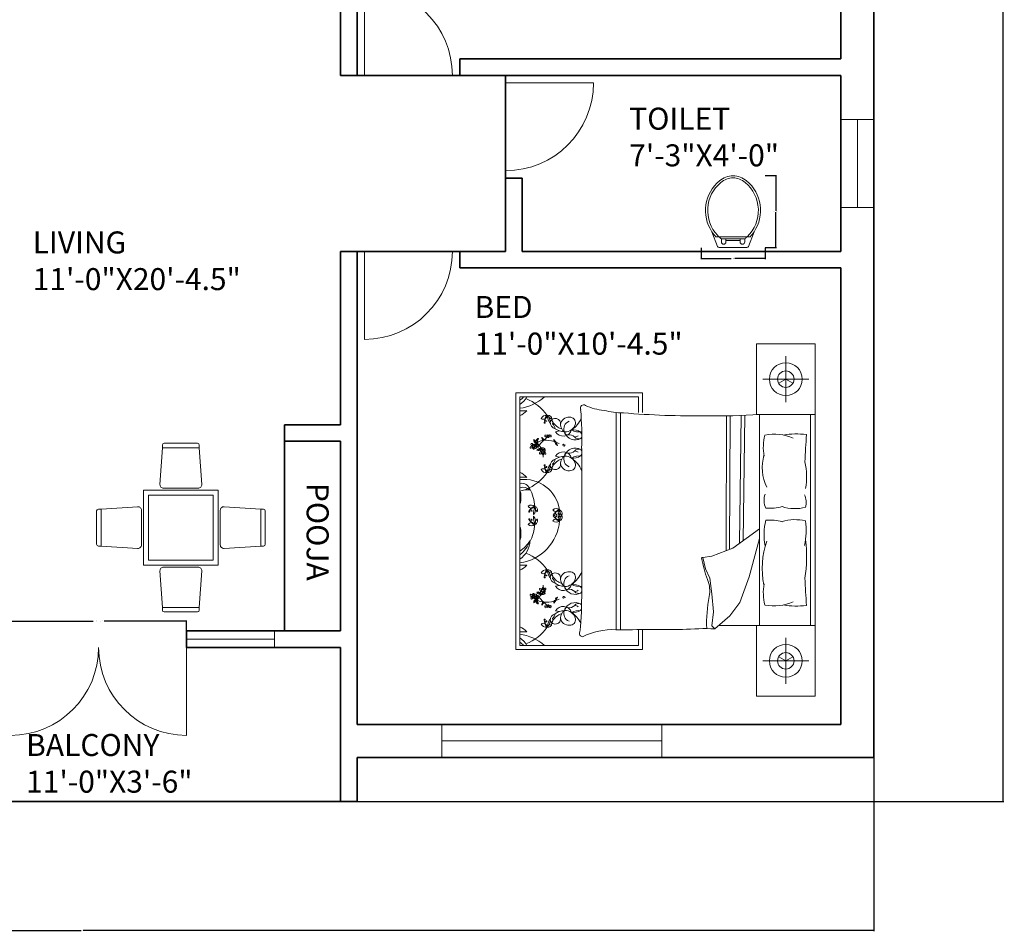
# Model space of a CAD drawing. Units: inches. Extents: x -59 to 444, y -680 to 63.
# Tile 2 of 9: x 176 to 444, y -680 to -431. Entities that reach past the tile are written whole.
import ezdxf

# ---------------------------------------------------------------- set-up
doc = ezdxf.new("R2010")
doc.units = ezdxf.units.IN
doc.header["$MEASUREMENT"] = 0
for name, color, linetype, lineweight in [('A-ANNO-DIMS', 2, 'Continuous', 18), ('A-AREA-IDEN', 7, 'Continuous', 18), ('A-DOOR', 3, 'Continuous', 18), ('A-FLOR-FIXT', 9, 'Continuous', 18), ('A-FURN', 8, 'Continuous', 13), ('A-GLAZ', 4, 'Continuous', 18), ('A-WALL', 7, 'Continuous', 35)]:
    doc.layers.add(name, color=color, linetype=linetype, lineweight=lineweight)
doc.styles.get("Standard").update_dxf_attribs({"font": 'arial.ttf'})
doc.dimstyles.get("Standard").update_dxf_attribs({"dimtxt": 0.18, "dimasz": 0.18, "dimexe": 0.18, "dimexo": 0.0625, "dimgap": 0.09, "dimtad": 0, "dimtih": 1, "dimtoh": 1, "dimdec": 0, "dimzin": 0, "dimdsep": 46, "dimlunit": 3, "dimtxsty": 'Standard', "dimcen": 0.09, "dimadec": 0, "dimazin": 0, "dimtfac": 1, "dimtdec": 0, "dimtofl": 0, "dimtmove": 0, "dimatfit": 3, "dimfxl": 1, "dimtolj": 1, "dimtzin": 0, "dimarcsym": 0})

# ---------------------------------------------------------------- blocks, each defined once
blk = doc.blocks.new('BED-SET-82')
for p, q in [((81.66, 0), (81.66, 96.02)), ((73.65, 80.14), (73.65, 92.69)), ((67.38, 86.42), (79.93, 86.42)), ((0, 82.67), (0, 12.67)), ((34.59, 82.67), (0, 82.67)), ((1.11, 81.56), (33.48, 81.56)), ((1.11, 13.79), (1.11, 81.56)), ((33.48, 81.56), (33.48, 77.33)), ((34.59, 77.35), (34.59, 82.67)), ((27.4, 77.34), (27.4, 18.1)), ((28.6, 77.25), (28.6, 18.1)), ((57.5, 76.47), (57.35, 39.63)), ((58.49, 76.47), (58.34, 40.01)), ((61.51, 76.52), (61.02, 41.65)), ((62.49, 76.56), (62.01, 42.37)), ((66.48, 19.2), (66.48, 76.81)), ((80.42, 76.81), (80.42, 19.2)), ((10.85, 72.1), (11.93, 72.31)), ((17.97, 67.5), (17.97, 28.52)), ((10.85, 65.39), (11.93, 65.18)), ((66.48, 45.58), (59.16, 40.32)), ((63.63, 32.54), (66.48, 43.01)), ((59.16, 40.32), (53.52, 38.18)), ((53.52, 38.18), (51, 37.79)), ((51, 37.79), (51.77, 34.68)), ((51.77, 34.68), (52.94, 32.15)), ((61.1, 25.54), (63.63, 32.54)), ((10.85, 29.96), (11.93, 30.17)), ((52.94, 32.15), (53.52, 27.87)), ((53.52, 27.87), (53.91, 23.01)), ((58.38, 21.84), (61.1, 25.54)), ((10.85, 23.25), (11.93, 23.04)), ((53.91, 23.01), (53.52, 19.12)), ((54.3, 18.34), (58.38, 21.84)), ((53.52, 19.12), (54.3, 18.34)), ((81.66, 19.2), (55.3, 19.2)), ((33.48, 18.1), (33.48, 13.79)), ((34.59, 12.67), (34.59, 18.1)), ((33.48, 13.79), (1.11, 13.79)), ((73.65, 15.87), (73.65, 3.33)), ((0, 12.67), (34.59, 12.67)), ((67.38, 9.6), (79.93, 9.6))]:
    blk.add_line(p, q)
for points in [[(81.66, 76.81), (65.65, 76.81), (65.65, 96.02), (81.66, 96.02)], [(73.65, 86.42), (71.71, 85.3)], [(73.65, 86.42), (75.6, 85.3)], [(65.65, 19.2), (65.65, 0), (81.66, 0)], [(73.65, 9.6), (71.71, 10.72)], [(73.65, 9.6), (75.6, 10.72)]]:
    blk.add_lwpolyline(points)
for points in [[(29.36, 77.22, -0.056112), (24.07, 77.92, -0.095341), (18.98, 79.27)], [(79.26, 71.3, 0.074897), (72.99, 71.18, -0.472817)], [(72.64, 51.66, 0.14099), (79.04, 51.47, 0.235245)], [(72.64, 47.56, -0.14099), (79.04, 47.75, -0.235245)], [(79.26, 24.72, -0.074897), (72.99, 24.83, 0.472817)], [(45.51, 18.14, -0.001242), (27.29, 18.1, 0.127202), (18.21, 16.17)]]:
    blk.add_lwpolyline(points, format="xyb")
for centre, radius in [((73.65, 86.42), 4.48), ((73.65, 86.42), 2.24), ((4.79, 68.15), 0.245), ((7.37, 66.55), 0.245), ((4.79, 27.2), 0.245), ((7.37, 28.8), 0.245), ((73.65, 9.6), 4.48), ((73.65, 9.6), 2.24)]:
    blk.add_circle(centre, radius)
for centre, radius, start, end in [((-2.26, 84.61), 6.11, 303.4617, 330.1116), ((-3.4, 86.8), 7.61, 306.3036, 316.4814), ((-0.58, 90.9), 12.54, 277.745, 311.8856), ((-1.82, 69.44), 12.54, 34.3865, 68.5908), ((18.5, 78.54), 0.875, 56.1736, 203.4781), ((-75.42, 70.44), 93.43, 358.1965, 4.7598), ((-0.84, 81.18), 5.1, 292.5547, 318.9546), ((1.9, 95.15), 17.35, 267.4081, 273.6519), ((8.23, 75.17), 1.39, 77.7115, 159.0387), ((7.48, 76.56), 1.05, 238.4633, 358.2869), ((10.92, 74.44), 3.17, 138.8402, 177.9352), ((9.01, 75.62), 1.03, 117.6827, 223.7762), ((8.78, 75.52), 1.04, 2.9516, 103.728), ((17.09, 78.43), 8.77, 192.5173, 207.1824), ((7.37, 74.92), 1.98, 345.4653, 54.2343), ((10.36, 77.64), 2.14, 211.3827, 255.2969), ((10.77, 74.3), 1.44, 350.264, 160.8688), ((9.21, 74.59), 0.883, 333.9755, 53.2681), ((14.47, 73.77), 2.29, 84.9449, 172.8857), ((14.7, 74.43), 1.62, 354.4856, 91.0538), ((11.21, 78.67), 7.27, 303.6671, 336.3547), ((48.48, 301.47), 225.05, 265.1265, 270.8855), ((54.75, 248.94), 172.53, 269.0718, 273.9), ((7.9, 74.55), 0.156, 177.9352, 11.4834), ((7.98, 74.56), 0.0756, 11.4834, 127.9409), ((8.42, 75.02), 0.0817, 223.7729, 159.7333), ((11.2, 74.64), 1.8, 175.969, 254.3045), ((8.81, 72.7), 1.92, 6.1662, 51.5825), ((13.94, 77.15), 4.53, 211.2614, 251.7045), ((13.58, 77.2), 5.15, 236.2883, 266.5076), ((12.92, 73.29), 2.39, 209.9085, 343.1337), ((14.98, 74.17), 2.79, 182.3591, 234.0401), ((15.34, 72.87), 2.23, 111.5819, 201.4221), ((13.5, 74.93), 2.89, 265.2933, 346.921), ((17.26, 76), 3.98, 238.8218, 280.751), ((15.53, 68.93), 3.7, 55.785, 94.7304), ((5.15, 69.73), 0.273, 124.3538, 214.3923), ((5.73, 69.92), 0.739, 176.9701, 248.2913), ((11.01, 73.81), 7.14, 212.6784, 216.3746), ((6.16, 69.54), 0.637, 122.8155, 187.3992), ((6.44, 69.46), 0.739, 109.4799, 177.6828), ((6.04, 69.93), 0.273, 56.8636, 146.9021), ((12.05, 66.08), 7.14, 145.1882, 148.8844), ((9.85, 70.48), 2.71, 178.3264, 187.1302), ((6.92, 70.1), 0.504, 11.3256, 64.4621), ((8.63, 70.83), 1.52, 190.2588, 210.656), ((7.62, 70.21), 0.461, 188.3432, 274.2869), ((8.02, 70.46), 0.805, 210.656, 242.6341), ((8.63, 71.15), 1.54, 218.2101, 226.3071), ((7.49, 69.86), 0.196, 325.7657, 67.4417), ((1.42, 76.4), 9.12, 313.1541, 322.0459), ((8.12, 70.92), 0.188, 142.4737, 265.053), ((8.37, 70.96), 0.404, 127.7621, 169.0403), ((8.15, 71.3), 0.568, 265.053, 338.3618), ((8.91, 70.52), 0.742, 113.4276, 137.6104), ((8.82, 71.29), 0.245, 183.2768, 356.7232), ((9, 70.85), 0.4, 139.7889, 227.6792), ((8.87, 70.71), 0.211, 227.6792, 350.3487), ((8.06, 70.86), 0.801, 353.0852, 15.7171), ((8.58, 70.76), 0.506, 350.3487, 43.6538), ((9.52, 71.28), 0.588, 198.7263, 262.5032), ((9.05, 71.01), 0.234, 1.1081, 91.8675), ((9.49, 70.88), 0.189, 255.2356, 54.9248), ((9.2, 70.95), 0.408, 11.5637, 52.6358), ((13.08, 69.9), 2.71, 178.3264, 187.1302), ((10.15, 69.53), 0.504, 11.3256, 64.4621), ((11.87, 70.25), 1.52, 190.2588, 210.656), ((13.92, 71.78), 0.596, 167.3041, 285.1471), ((15.53, 68.93), 3.7, 122.7011, 126.3445), ((16.23, 72.92), 3.06, 199.2822, 299.1751), ((14.59, 69.3), 1.97, 41.5653, 105.1471), ((15.67, 73.38), 2.76, 277.436, 299.9149), ((17.14, 71.56), 1.44, 221.5653, 293.8354), ((16.91, 71.07), 1.16, 17.4186, 52.325), ((16.91, 71.07), 1.16, 314.4517, 343.3657), ((80.39, 67.87), 12.87, 165.1039, 191.0369), ((70.47, 59.07), 12.38, 65.1316, 101.7583), ((993.04, 18.37), 915.3, 176.68521, 177.14978), ((4.09, 67.78), 0.188, 142.4737, 265.053), ((4.34, 67.82), 0.404, 61.2196, 169.0403), ((4.12, 68.16), 0.568, 265.053, 338.3618), ((4.6, 68.65), 0.483, 157.4086, 261.4386), ((4.33, 68.67), 0.242, 58.0499, 135.6268), ((4.88, 67.38), 0.742, 113.4276, 137.6104), ((4.58, 68.51), 0.162, 172.906, 277.132), ((4.05, 68.22), 0.771, 14.7558, 58.0499), ((4.97, 67.71), 0.4, 139.7889, 227.6792), ((4.84, 67.57), 0.211, 227.6792, 350.3487), ((5.13, 68.42), 0.333, 36.1046, 181.4281), ((4.03, 67.71), 0.801, 353.0852, 15.7171), ((5.55, 69.69), 0.637, 190.3057, 287.1958), ((4.55, 67.62), 0.506, 350.3487, 43.6538), ((5.49, 68.14), 0.588, 198.7263, 262.5032), ((4.94, 68.68), 0.337, 270.0645, 331.1507), ((5.22, 68.6), 0.385, 221.8413, 265.7877), ((5.02, 67.87), 0.234, 1.1081, 91.8675), ((5.22, 68.46), 0.24, 263.7526, 41.7054), ((5.17, 67.81), 0.408, 11.5637, 86.365), ((5.48, 69.74), 0.283, 216.3746, 291.7548), ((7.98, 65.77), 3.99, 124.0033, 132.4917), ((5.46, 67.74), 0.189, 255.2356, 54.9248), ((3.88, 65.27), 4.26, 63.7819, 68.2913), ((6.16, 68.55), 0.678, 128.3208, 208.8162), ((6.28, 68.6), 0.81, 207.7043, 254.3516), ((5.67, 69.28), 0.213, 289.3605, 111.7548), ((5.83, 69.28), 0.213, 221.8703, 44.2646), ((6.79, 68.66), 1.11, 157.2305, 229.0635), ((6.42, 69.03), 0.656, 174.4544, 220.6188), ((5.75, 68.13), 1.11, 270.278, 342.111), ((6.5, 66.74), 0.788, 98.7227, 159.3375), ((2.69, 65.36), 4.78, 30.544, 49.818), ((6.18, 69.63), 0.283, 148.8844, 224.2646), ((5.32, 68.09), 0.788, 340.0041, 40.6188), ((7.98, 65.77), 3.99, 94.756, 119.2041), ((16.47, 60.04), 13.12, 132.2412, 142.1744), ((6.28, 68.17), 0.656, 278.7227, 324.8872), ((6.16, 67.64), 0.678, 290.5253, 358.5375), ((7.18, 67.05), 0.483, 157.4086, 261.4386), ((6.91, 67.07), 0.242, 58.0499, 135.6268), ((7.48, 67.83), 0.678, 182.8499, 266.1226), ((7.22, 68.31), 0.656, 231.7607, 277.9252), ((7.73, 68.42), 1.11, 214.5369, 286.3699), ((6.63, 66.62), 0.771, 14.7558, 58.0499), ((2.69, 65.36), 4.78, 23.0501, 23.8477), ((7.42, 66.88), 0.788, 37.3105, 97.9252), ((7.71, 66.82), 0.333, 36.1046, 181.4281), ((7.51, 67.96), 0.81, 265.0106, 311.658), ((8.18, 61.81), 7.95, 73.5842, 93.8277), ((10.85, 69.64), 0.461, 188.3432, 274.2869), ((11.25, 69.89), 0.805, 210.656, 242.6341), ((11.86, 70.58), 1.54, 218.2101, 226.3071), ((10.72, 69.29), 0.196, 325.7657, 67.4417), ((11.27, 68.93), 0.461, 147.5332, 233.4768), ((11.69, 69.16), 0.805, 179.1859, 211.164), ((10.9, 68.98), 0.196, 354.3784, 96.0543), ((8.18, 61.81), 7.95, 63.0032, 69.8941), ((12.3, 69.53), 1.52, 211.164, 231.5612), ((12.56, 70.77), 2.71, 234.6898, 243.4936), ((12.58, 69.37), 1.54, 195.5129, 203.6099), ((10.85, 68.37), 0.504, 357.3579, 50.4944), ((13.02, 68.47), 0.185, 12.7051, 190.4384), ((13.13, 68.49), 0.301, 190.4384, 10.4136), ((16.23, 64.57), 3.06, 60.8249, 160.7178), ((17.14, 65.93), 1.44, 66.1646, 138.4347), ((16.91, 66.41), 1.16, 23.2856, 45.5483), ((6.1, 67.75), 0.81, 244.9899, 291.6373), ((6.67, 66.18), 0.188, 142.4737, 265.053), ((6.91, 66.22), 0.404, 61.2196, 169.0403), ((6.7, 66.56), 0.568, 265.053, 338.3618), ((7.45, 65.78), 0.742, 113.4276, 137.6104), ((7.16, 66.91), 0.162, 172.906, 277.132), ((7.55, 66.11), 0.4, 139.7889, 227.6792), ((7.42, 65.97), 0.211, 227.6792, 350.3487), ((6.6, 66.12), 0.801, 353.0852, 15.7171), ((2.69, 65.36), 4.78, 357.1071, 4.7585), ((7.13, 66.02), 0.506, 350.3487, 43.6538), ((7.51, 67.08), 0.337, 270.0645, 331.1507), ((7.8, 67), 0.385, 221.8413, 265.7877), ((8.07, 66.54), 0.588, 198.7263, 262.5032), ((7.6, 66.27), 0.234, 1.1081, 91.8675), ((7.8, 66.86), 0.24, 263.7526, 41.7054), ((7.75, 66.21), 0.408, 11.5637, 86.365), ((8.04, 66.14), 0.189, 255.2356, 54.9248), ((11.2, 62.85), 1.8, 105.6955, 184.031), ((8.81, 64.79), 1.92, 308.4175, 353.8338), ((13.94, 60.34), 4.53, 108.2955, 148.7386), ((13.58, 60.29), 5.15, 93.4924, 123.7117), ((12.92, 64.2), 2.39, 16.8663, 150.0915), ((14.98, 63.32), 2.79, 125.9599, 177.6409), ((15.34, 64.62), 2.23, 158.5779, 248.4181), ((13.5, 62.56), 2.89, 13.079, 94.7067), ((13.92, 65.71), 0.596, 74.8529, 192.6959), ((15.53, 68.56), 3.7, 233.6555, 237.2989), ((14.59, 68.19), 1.97, 254.8529, 318.4347), ((17.26, 61.49), 3.98, 79.7133, 121.1782), ((15.53, 68.56), 3.7, 265.2696, 304.215), ((11.21, 58.82), 7.27, 21.4941, 56.3329), ((15.67, 64.11), 2.76, 60.0851, 82.564), ((16.91, 66.41), 1.16, 307.675, 336.7144), ((79.44, 62.32), 12.22, 163.8254, 206.1239), ((7.48, 60.93), 1.05, 1.7131, 121.5367), ((8.23, 62.32), 1.39, 200.9613, 282.2885), ((7.9, 62.94), 0.156, 348.5166, 182.0648), ((10.92, 63.05), 3.17, 182.0648, 221.1598), ((7.98, 62.92), 0.0756, 232.0591, 348.5166), ((9.01, 61.87), 1.03, 136.2238, 242.3173), ((8.36, 62.49), 0.136, 200.2817, 136.2238), ((7.37, 62.57), 1.98, 305.7657, 14.5347), ((17.09, 59.06), 8.77, 152.8176, 167.4827), ((8.78, 61.97), 1.04, 256.272, 357.0484), ((10.36, 59.85), 2.14, 104.7031, 148.6173), ((10.77, 63.19), 1.44, 199.1312, 9.736), ((9.21, 62.9), 0.883, 306.7319, 26.0245), ((14.47, 63.72), 2.29, 187.1143, 275.0551), ((14.7, 63.06), 1.62, 268.9462, 5.5144), ((62.46, 59.9), 16.88, 348.8159, 13.6573), ((-0.84, 56.3), 5.1, 41.0454, 67.4453), ((1.9, 42.34), 17.35, 86.3481, 92.5919), ((2.32, 49.39), 9.7, 8.1803, 97.1364), ((-1.82, 68.04), 12.54, 291.4092, 325.6135), ((1.64, 55.79), 2.25, 10.9261, 103.6102), ((1.95, 54.1), 2.85, 48.0951, 107.1391), ((-7.29, 50.75), 12.54, 4.4623, 27.4146), ((-5.48, 54.26), 6.89, 343.5431, 17.0202), ((3.2, 50.64), 5.61, 83.3805, 111.883), ((72.82, 53.43), 5.09, 161.4593, 204.9817), ((74.48, 52.78), 4.75, 343.8974, 26.6563), ((-9.03, 51.53), 10.2, 4.3787, 5.6357), ((-16.02, 46.16), 18.22, 19.7217, 19.9028), ((4.27, 50.7), 1.39, 47.7873, 129.1145), ((4.32, 52.28), 1.05, 208.5391, 328.3627), ((6.24, 48.73), 3.17, 108.9159, 148.011), ((5.17, 50.7), 1.03, 87.7585, 193.852), ((13.58, 49.1), 8.77, 162.593, 177.2582), ((3.4, 50.91), 1.98, 315.5411, 24.3101), ((7.35, 51.78), 2.14, 181.4585, 225.3727), ((4.92, 50.73), 1.04, 333.0274, 73.8037), ((10.99, 49.74), 1.39, 47.7873, 129.1145), ((69.43, 62.98), 11.76, 264.0129, 285.8293), ((3.68, 50.33), 0.156, 148.011, 341.5592), ((3.68, 48.22), 0.156, 18.4408, 211.989), ((3.75, 50.3), 0.0756, 341.5592, 98.0167), ((4.36, 50.48), 0.0817, 193.9791, 129.8091), ((13.58, 49.44), 8.77, 182.7418, 197.407), ((3.4, 47.64), 1.98, 335.6899, 44.4589), ((11.03, 51.32), 1.05, 208.5391, 328.3627), ((10.39, 49.37), 0.156, 148.011, 341.5592), ((10.39, 49.18), 0.156, 18.4408, 211.989), ((12.95, 47.77), 3.17, 108.9159, 148.011), ((12.95, 50.78), 3.17, 211.989, 251.0841), ((10.47, 49.34), 0.0756, 341.5592, 98.0167), ((10.47, 49.21), 0.0756, 261.9833, 18.4408), ((11.88, 49.74), 1.03, 87.7585, 193.852), ((11.88, 48.8), 1.03, 166.148, 272.2415), ((11.02, 49.02), 0.136, 230.0755, 166.148), ((11.07, 49.52), 0.0817, 193.9791, 129.8091), ((10.12, 49.95), 1.98, 315.5411, 24.3101), ((20.29, 48.14), 8.77, 162.593, 177.2582), ((10.12, 48.6), 1.98, 335.6899, 44.4589), ((20.29, 50.4), 8.77, 182.7418, 197.407), ((11.63, 49.77), 1.04, 333.0274, 73.8037), ((14.06, 50.82), 2.14, 181.4585, 225.3727), ((11.63, 48.78), 1.04, 286.1963, 26.9726), ((14.06, 47.73), 2.14, 134.6273, 178.5415), ((-0.58, 48.76), 12.54, 277.745, 355.5377), ((-5.48, 44.29), 6.89, 342.9798, 16.4569), ((-9.03, 47.02), 10.2, 354.3643, 355.6213), ((-16.02, 52.39), 18.22, 340.0972, 340.2783), ((4.32, 46.27), 1.05, 31.6373, 151.4609), ((4.27, 47.85), 1.39, 230.8855, 312.2127), ((6.24, 49.82), 3.17, 211.989, 251.0841), ((3.75, 48.25), 0.0756, 261.9833, 18.4408), ((-7.29, 47.8), 12.54, 332.5854, 355.5377), ((5.17, 47.84), 1.03, 166.148, 272.2415), ((4.3, 48.06), 0.136, 230.0755, 166.148), ((7.35, 46.76), 2.14, 134.6273, 178.5415), ((4.92, 47.82), 1.04, 286.1963, 26.9726), ((11.03, 47.23), 1.05, 31.6373, 151.4609), ((10.99, 48.81), 1.39, 230.8855, 312.2127), ((84.66, 43.95), 16.93, 166.3762, 190.1383), ((69.43, 36.24), 11.76, 74.1707, 95.9871), ((62.12, 45.23), 17.11, 346.04, 8.4751), ((-2.26, 42.46), 6.11, 303.4617, 358.728), ((-5.54, 48.66), 11.33, 305.947, 325.9877), ((-3.4, 44.66), 7.61, 306.3036, 342.1496), ((89.53, 34.92), 22.32, 160.7385, 191.9603), ((44.52, 37.87), 34.82, 350.503, 7.7804), ((-1.82, 27.3), 12.54, 34.3865, 68.5908), ((50.92, 37.57), 0.232, 70.2464, 181.1377), ((1.9, 53.01), 17.35, 267.4081, 273.6519), ((-0.84, 39.04), 5.1, 292.5547, 318.9546), ((87.28, 44.46), 37.24, 190.6617, 199.8806), ((8.23, 33.03), 1.39, 77.7115, 159.0387), ((7.48, 34.42), 1.05, 238.4633, 358.2869), ((10.92, 32.3), 3.17, 138.8402, 177.9352), ((7.9, 32.41), 0.156, 177.9352, 11.4834), ((7.98, 32.42), 0.0756, 11.4834, 127.9409), ((9.01, 33.48), 1.03, 117.6827, 223.7762), ((8.42, 32.88), 0.0817, 223.7729, 159.7333), ((8.78, 33.38), 1.04, 2.9516, 103.728), ((10.36, 35.5), 2.14, 211.3827, 255.2969), ((7.37, 32.78), 1.98, 345.4653, 54.2343), ((17.09, 36.29), 8.77, 192.5173, 207.1824), ((11.2, 32.5), 1.8, 175.969, 254.3045), ((10.77, 32.15), 1.44, 350.264, 160.8688), ((9.21, 32.45), 0.883, 333.9755, 53.2681), ((13.94, 35.01), 4.53, 211.2614, 251.7045), ((14.47, 31.63), 2.29, 84.9449, 172.8857), ((15.34, 30.72), 2.23, 111.5819, 201.4221), ((14.7, 32.29), 1.62, 354.4856, 91.0538), ((11.21, 36.52), 7.27, 303.6671, 338.5059), ((7.42, 29.38), 0.211, 9.6513, 132.3208), ((2.69, 29.98), 4.78, 355.2415, 2.8929), ((8.81, 30.56), 1.92, 6.1662, 51.5825), ((13.58, 35.05), 5.15, 236.2883, 266.5076), ((12.92, 31.15), 2.39, 209.9085, 343.1337), ((14.98, 32.03), 2.79, 182.3591, 234.0401), ((13.5, 32.79), 2.89, 265.2933, 346.921), ((13.92, 29.64), 0.596, 167.3041, 285.1471), ((15.53, 26.79), 3.7, 122.7011, 126.3445), ((16.23, 30.78), 3.06, 199.2822, 299.1751), ((17.26, 33.86), 3.98, 238.8218, 280.2867), ((15.53, 26.79), 3.7, 55.785, 94.7304), ((16.91, 28.93), 1.16, 23.2856, 52.325), ((45.11, 28.65), 7.82, 348.6608, 23.7384), ((80.39, 28.14), 12.87, 168.9631, 194.8961), ((993.04, 77.64), 915.3, 182.85022, 183.31479), ((4.09, 27.57), 0.188, 94.947, 217.5263), ((4.34, 27.53), 0.404, 190.9597, 298.7804), ((4.12, 27.19), 0.568, 21.6382, 94.947), ((4.6, 26.7), 0.483, 98.5614, 202.5914), ((4.88, 27.96), 0.742, 222.3896, 246.5724), ((4.58, 26.83), 0.162, 82.868, 187.094), ((4.05, 27.13), 0.771, 301.9501, 345.2442), ((4.97, 27.64), 0.4, 132.3208, 220.2111), ((4.84, 27.78), 0.211, 9.6513, 132.3208), ((4.03, 27.63), 0.801, 344.2829, 6.9148), ((5.13, 26.93), 0.333, 178.5719, 323.8954), ((4.55, 27.73), 0.506, 316.3462, 9.6513), ((5.49, 27.21), 0.588, 97.4968, 161.2737), ((5.22, 26.74), 0.385, 94.2123, 138.1587), ((4.94, 26.66), 0.337, 28.8493, 89.9355), ((5.02, 27.48), 0.234, 268.1325, 358.8919), ((5.17, 27.53), 0.408, 273.635, 348.4363), ((5.22, 26.89), 0.24, 318.2946, 96.2474), ((5.46, 27.61), 0.189, 305.0752, 104.7644), ((6.16, 26.8), 0.678, 151.1838, 231.6792), ((6.28, 26.75), 0.81, 105.6484, 152.2957), ((6.79, 26.69), 1.11, 130.9365, 202.7695), ((6.1, 27.59), 0.81, 68.3627, 115.0101), ((5.75, 27.21), 1.11, 17.889, 89.722), ((6.5, 28.61), 0.788, 200.6625, 261.2773), ((2.69, 29.98), 4.78, 310.182, 329.456), ((5.32, 27.26), 0.788, 319.3812, 19.9959), ((16.47, 35.31), 13.12, 217.8256, 227.7588), ((6.28, 27.18), 0.656, 35.1128, 81.2773), ((6.16, 27.71), 0.678, 1.4625, 69.4747), ((6.67, 29.17), 0.188, 94.947, 217.5263), ((6.91, 29.13), 0.404, 190.9597, 298.7804), ((6.7, 28.79), 0.568, 21.6382, 94.947), ((7.18, 28.3), 0.483, 98.5614, 202.5914), ((6.91, 28.28), 0.242, 224.3732, 301.9501), ((7.48, 27.52), 0.678, 93.8774, 177.1501), ((7.73, 26.92), 1.11, 73.6301, 145.4631), ((7.22, 27.04), 0.656, 82.0748, 128.2393), ((7.45, 29.56), 0.742, 222.3896, 246.5724), ((7.16, 28.43), 0.162, 82.868, 187.094), ((6.63, 28.73), 0.771, 301.9501, 345.2442), ((2.69, 29.98), 4.78, 336.1523, 336.9499), ((7.55, 29.24), 0.4, 132.3208, 220.2111), ((7.42, 28.47), 0.788, 262.0748, 322.6895), ((6.6, 29.23), 0.801, 344.2829, 6.9148), ((7.71, 28.53), 0.333, 178.5719, 323.8954), ((7.51, 27.39), 0.81, 48.342, 94.9894), ((7.13, 29.33), 0.506, 316.3462, 9.6513), ((8.07, 28.81), 0.588, 97.4968, 161.2737), ((7.8, 28.34), 0.385, 94.2123, 138.1587), ((7.51, 28.26), 0.337, 28.8493, 89.9355), ((7.6, 29.08), 0.234, 268.1325, 358.8919), ((7.75, 29.13), 0.408, 273.635, 348.4363), ((7.8, 28.49), 0.24, 318.2946, 96.2474), ((8.04, 29.21), 0.189, 305.0752, 104.7644), ((12.3, 25.81), 1.52, 128.4388, 148.836), ((12.56, 24.58), 2.71, 116.5064, 125.3102), ((10.85, 26.98), 0.504, 309.5056, 2.6421), ((13.13, 26.86), 0.301, 349.5864, 169.5616), ((13.02, 26.88), 0.185, 169.5616, 347.2949), ((14.59, 27.16), 1.97, 41.5653, 105.1471), ((15.67, 31.24), 2.76, 277.436, 299.9149), ((17.14, 29.42), 1.44, 221.5653, 293.8354), ((-81.98, 27.37), 99.96, 354.3113, 0.6567), ((16.91, 28.93), 1.16, 314.4517, 336.771), ((88.3, 19.99), 36.24, 168.6608, 182.5481), ((4.33, 26.68), 0.242, 224.3732, 301.9501), ((5.15, 25.62), 0.273, 145.6077, 235.6462), ((5.55, 25.66), 0.637, 72.8042, 169.6943), ((5.73, 25.43), 0.739, 111.7087, 183.0299), ((11.01, 21.54), 7.14, 143.6254, 147.3216), ((5.48, 25.6), 0.283, 68.2452, 143.6254), ((7.98, 29.57), 3.99, 227.5083, 235.9967), ((3.88, 30.08), 4.26, 291.7087, 296.2181), ((6.16, 25.8), 0.637, 172.6008, 237.1845), ((5.67, 26.07), 0.213, 248.2452, 70.6395), ((5.83, 26.07), 0.213, 315.7354, 138.1297), ((6.44, 25.88), 0.739, 182.3172, 250.5201), ((6.42, 26.32), 0.656, 139.3812, 185.5456), ((6.04, 25.42), 0.273, 213.0979, 303.1364), ((6.18, 25.72), 0.283, 135.7354, 211.1156), ((12.05, 29.27), 7.14, 211.1156, 214.8118), ((7.98, 29.57), 3.99, 240.7959, 265.244), ((8.63, 24.52), 1.52, 149.344, 169.7412), ((9.85, 24.87), 2.71, 172.8698, 181.6736), ((6.92, 25.25), 0.504, 295.5379, 348.6744), ((7.62, 25.14), 0.461, 85.7131, 171.6568), ((8.02, 24.88), 0.805, 117.3659, 149.344), ((8.63, 24.19), 1.54, 133.6929, 141.7899), ((7.49, 25.49), 0.196, 292.5583, 34.2343), ((8.18, 33.53), 7.95, 266.1723, 286.4158), ((1.42, 18.95), 9.12, 37.9541, 46.8459), ((8.12, 24.43), 0.188, 94.947, 217.5263), ((8.37, 24.39), 0.404, 190.9597, 232.2379), ((8.15, 24.05), 0.568, 21.6382, 94.947), ((8.91, 24.82), 0.742, 222.3896, 246.5724), ((8.82, 24.05), 0.245, 3.2768, 176.7232), ((9, 24.5), 0.4, 132.3208, 220.2111), ((8.87, 24.64), 0.211, 9.6513, 132.3208), ((8.06, 24.49), 0.801, 344.2829, 6.9148), ((8.58, 24.59), 0.506, 316.3462, 9.6513), ((9.52, 24.07), 0.588, 97.4968, 161.2737), ((9.05, 24.34), 0.234, 268.1325, 358.8919), ((9.49, 24.47), 0.189, 305.0752, 104.7644), ((9.2, 24.39), 0.408, 307.3642, 348.4363), ((11.87, 25.09), 1.52, 149.344, 169.7412), ((13.08, 25.44), 2.71, 172.8698, 181.6736), ((10.15, 25.82), 0.504, 295.5379, 348.6744), ((10.85, 25.71), 0.461, 85.7131, 171.6568), ((11.25, 25.46), 0.805, 117.3659, 149.344), ((11.86, 24.77), 1.54, 133.6929, 141.7899), ((10.72, 26.06), 0.196, 292.5583, 34.2343), ((11.27, 26.42), 0.461, 126.5232, 212.4668), ((12.92, 22.06), 2.39, 16.8663, 150.0915), ((11.69, 26.18), 0.805, 148.836, 180.8141), ((10.9, 26.37), 0.196, 263.9457, 5.6216), ((8.18, 33.53), 7.95, 290.1059, 296.9968), ((12.58, 25.97), 1.54, 156.3901, 164.4871), ((16.23, 22.43), 3.06, 60.8249, 160.7178), ((14.59, 26.04), 1.97, 254.8529, 318.4347), ((15.67, 21.97), 2.76, 60.0851, 82.564), ((17.14, 23.79), 1.44, 66.1646, 138.4347), ((16.91, 24.27), 1.16, 26.442, 45.5483), ((70.47, 36.95), 12.38, 258.2417, 294.8684), ((11.2, 20.71), 1.8, 105.6955, 184.031), ((8.81, 22.64), 1.92, 308.4175, 353.8338), ((13.94, 18.19), 4.53, 108.2955, 148.7386), ((13.58, 18.15), 5.15, 93.4924, 123.7117), ((14.98, 21.18), 2.79, 125.9599, 177.6409), ((15.34, 22.48), 2.23, 158.5779, 248.4181), ((13.5, 20.42), 2.89, 13.079, 94.7067), ((13.92, 23.57), 0.596, 74.8529, 192.6959), ((15.53, 26.42), 3.7, 233.6555, 237.2989), ((17.26, 19.35), 3.98, 80.8446, 121.1782), ((15.53, 26.42), 3.7, 265.2696, 304.215), ((11.21, 16.68), 7.27, 26.7003, 56.3329), ((16.91, 24.27), 1.16, 307.675, 329.9707), ((-0.84, 14.16), 5.1, 41.0454, 67.4453), ((-1.82, 25.9), 12.54, 291.4092, 325.6135), ((7.48, 18.79), 1.05, 1.7131, 121.5367), ((8.23, 20.18), 1.39, 200.9613, 282.2885), ((7.9, 20.8), 0.156, 348.5166, 182.0648), ((10.92, 20.91), 3.17, 182.0648, 221.1598), ((7.98, 20.78), 0.0756, 232.0591, 348.5166), ((9.01, 19.73), 1.03, 136.2238, 242.3173), ((8.36, 20.35), 0.136, 200.2817, 136.2238), ((17.09, 16.92), 8.77, 152.8176, 167.4827), ((7.37, 20.43), 1.98, 305.7657, 14.5347), ((10.36, 17.71), 2.14, 104.7031, 148.6173), ((8.78, 19.83), 1.04, 256.272, 357.0484), ((10.77, 21.05), 1.44, 199.1312, 9.736), ((9.21, 20.75), 0.883, 306.7319, 26.0245), ((14.47, 21.58), 2.29, 187.1143, 275.0551), ((14.7, 20.91), 1.62, 268.9462, 5.5144), ((1.9, 0.2), 17.35, 86.3481, 92.5919), ((-0.58, 4.45), 12.54, 48.1144, 82.255), ((18.27, 17.06), 0.886, 152.6588, 266.02), ((51.91, -69.69), 88.07, 88.447, 94.1706), ((-2.26, 10.74), 6.11, 29.8884, 56.5383), ((-3.4, 8.54), 7.61, 43.5186, 53.6964)]:
    blk.add_arc(centre, radius, start, end)
blk = doc.blocks.new('DINING-SET-4')
for p, q in [((27.54, 46.01), (18.47, 46.01)), ((17.3, 34.79), (17.98, 44.78)), ((17.98, 45.52), (17.98, 44.78)), ((28.03, 44.78), (17.98, 44.78)), ((28.03, 44.78), (28.03, 45.52)), ((28.03, 44.78), (28.7, 34.79)), ((18.28, 33.76), (27.73, 33.76)), ((0, 27.54), (0, 18.47)), ((1.22, 28.03), (0.49, 28.03)), ((1.22, 28.03), (11.22, 28.71)), ((1.22, 28.03), (1.22, 17.98)), ((12.25, 18.28), (12.25, 27.73)), ((33.76, 27.73), (33.76, 18.28)), ((34.79, 28.71), (44.78, 28.03)), ((45.52, 28.03), (44.78, 28.03)), ((44.78, 17.98), (44.78, 28.03)), ((46.01, 18.47), (46.01, 27.54)), ((0.49, 17.98), (1.22, 17.98)), ((11.22, 17.3), (1.22, 17.98)), ((44.78, 17.98), (34.79, 17.3)), ((44.78, 17.98), (45.52, 17.98)), ((17.98, 1.23), (17.3, 11.22)), ((27.73, 12.25), (18.28, 12.25)), ((28.7, 11.22), (28.03, 1.23)), ((17.98, 1.23), (28.03, 1.23)), ((17.98, 1.23), (17.98, 0.49)), ((18.47, 0), (27.54, 0)), ((28.03, 0.49), (28.03, 1.23))]:
    blk.add_line(p, q)
for points in [[(12.79, 12.8), (12.79, 33.21), (33.21, 33.21), (33.21, 12.8)], [(14.16, 14.16), (14.16, 31.85), (31.85, 31.85), (31.85, 14.16)]]:
    blk.add_lwpolyline(points, close=True)
for centre, radius, start, end in [((18.47, 45.52), 0.49, 90, 180), ((27.54, 45.52), 0.49, 0, 90), ((18.28, 34.74), 0.98, 176.8779, 270), ((27.73, 34.74), 0.98, 270, 3.1221), ((0.49, 27.54), 0.49, 90, 180), ((11.27, 27.73), 0.98, 0, 93.1221), ((34.74, 27.73), 0.98, 86.8779, 180), ((45.52, 27.54), 0.49, 0, 90), ((0.49, 18.47), 0.49, 180, 270), ((11.27, 18.28), 0.98, 266.8779, 0), ((34.74, 18.28), 0.98, 180, 273.1221), ((45.52, 18.47), 0.49, 270, 0), ((18.28, 11.27), 0.98, 90, 183.1221), ((27.73, 11.27), 0.98, 356.8779, 90), ((18.47, 0.49), 0.49, 180, 270), ((27.54, 0.49), 0.49, 270, 0)]:
    blk.add_arc(centre, radius, start, end)
blk = doc.blocks.new('WC-FLOOR')
for p, q in [((2.81, 2.97), (3.64, 2.97)), ((3.64, 2.97), (7.5, 2.97)), ((11.36, 2.97), (7.5, 2.97)), ((11.36, 2.97), (12.18, 2.97))]:
    blk.add_line(p, q)
for points in [[(1.75, 4.32, -0.383919), (3.81, 18.21, -0.163732), (7.5, 19.62, -0.359733)], [(3.24, 3.37, -0.431639), (4.18, 17.76, -0.162618), (7.5, 19.04, -0.470877)], [(13.24, 4.32, 0.383919), (11.19, 18.21, 0.163732), (7.5, 19.62, 0.359733)], [(11.36, 2.97, 0.448546), (10.81, 17.76, 0.162618), (7.5, 19.04, 0.470877)], [(2.81, 2.97, -0.040937), (1.75, 4.32, -0.163732)], [(7.5, 0), (3.75, 0, -0.31031), (3.29, 0.32), (1.75, 4.32, -0.209071)], [(3.64, 2.97, -0.014165), (3.24, 3.37, -0.162618)], [(4.31, 2.38, -0.022712), (3.64, 2.97, -0.162618)], [(7.5, 0), (11.24, 0, 0.31031), (11.7, 0.32), (13.24, 4.32, 0.209071)], [(10.68, 2.38, 0.022712), (11.36, 2.97, 0.162618)], [(12.18, 2.97, 0.040937), (13.24, 4.32, 0.163732)], [(7.5, 2.38), (4.31, 2.38, -0.022712)], [(4.31, 2.38), (4.31, 1.55, 1), (5.56, 1.55), (5.56, 1.98)], [(7.5, 2.38), (10.68, 2.38, 0.476108)], [(10.68, 2.38), (10.68, 1.55, -1), (9.43, 1.55), (9.43, 1.98)]]:
    blk.add_lwpolyline(points, format="xyb")
for points in [[(5.56, 1.98), (5.56, 2.38)], [(9.43, 1.98), (5.56, 1.98)], [(9.43, 1.98), (9.43, 2.38)]]:
    blk.add_lwpolyline(points)
blk = doc.blocks.new('WIN-60-W9')
for p, q in [((60, 9), (0, 9)), ((0, 9), (0, 0)), ((60, 0), (60, 9)), ((0, 4.5), (60, 4.5)), ((0, 0), (60, 0))]:
    blk.add_line(p, q)
blk = doc.blocks.new('WIN-24-W9')
for p, q in [((0, 24), (0, 0)), ((9, 24), (0, 24)), ((4.5, 24), (4.5, 0)), ((9, 0), (9, 24)), ((0, 0), (9, 0))]:
    blk.add_line(p, q)
blk = doc.blocks.new('WIN-24-W4-5')
for p, q in [((24, 4.5), (0, 4.5)), ((0, 4.5), (0, 0)), ((24, 0), (24, 4.5)), ((24, 2.25), (0, 2.25)), ((0, 0), (24, 0))]:
    blk.add_line(p, q)
blk = doc.blocks.new('DOOR-SWING-24')
blk.add_line((24, 0), (0, 0))
blk.add_arc((24, 0), 24, 90, 180)
blk = doc.blocks.new('DOOR-DOUBLE-48')
for p, q in [((0, 0), (0, 24)), ((48, 0), (48, 24))]:
    blk.add_line(p, q)
for centre, start, end in [((0, 0), 0, 90), ((48, 0), 90, 180)]:
    blk.add_arc(centre, 24, start, end)
blk = doc.blocks.new('*D18')
at = {"layer": 'A-ANNO-DIMS', "color": 0, "lineweight": -2, "transparency": 16777216}
for p, q in [((173.23, -602.37), (173.23, -595.06)), ((173.41, -595.24), (195.74, -595.24)), ((221.05, -595.24), (198.72, -595.24)), ((221.23, -602.37), (221.23, -595.06))]:
    blk.add_line(p, q, dxfattribs=at)
at = {"layer": 'A-ANNO-DIMS', "color": 0, "transparency": 16777216}
for points in [[(173.41, -595.21), (173.41, -595.27), (173.23, -595.24)], [(221.05, -595.21), (221.05, -595.27), (221.23, -595.24)]]:
    blk.add_solid(points, dxfattribs=at)
at = {"layer": 'Defpoints', "color": 0, "transparency": 16777216}
for p in [(173.23, -595.24), (173.23, -602.44), (221.23, -602.44)]:
    blk.add_point(p, dxfattribs=at)
at = {"layer": 'A-ANNO-DIMS', "color": 0, "transparency": 16777216, "insert": (197.23, -595.24), "char_height": 0.18, "attachment_point": 5}
blk.add_mtext('\\A1;DOUBLE DOOR 48 TYP.', dxfattribs=at)
blk = doc.blocks.new('*D30')
at = {"layer": 'A-ANNO-DIMS', "color": 0, "lineweight": -2, "transparency": 16777216}
for p, q in [((379.07, -473.77), (382.13, -473.77)), ((381.95, -473.95), (381.95, -483.4)), ((381.95, -493.22), (381.95, -483.77)), ((379.07, -493.4), (382.13, -493.4))]:
    blk.add_line(p, q, dxfattribs=at)
at = {"layer": 'A-ANNO-DIMS', "color": 0, "transparency": 16777216}
for points in [[(381.92, -473.95), (381.98, -473.95), (381.95, -473.77)], [(381.92, -493.22), (381.98, -493.22), (381.95, -493.4)]]:
    blk.add_solid(points, dxfattribs=at)
at = {"layer": 'Defpoints', "color": 0, "transparency": 16777216}
for p in [(379.01, -473.77), (381.95, -473.77), (379.01, -493.4)]:
    blk.add_point(p, dxfattribs=at)
at = {"layer": 'A-ANNO-DIMS', "color": 0, "transparency": 16777216, "insert": (381.95, -483.59), "char_height": 0.18, "attachment_point": 5}
blk.add_mtext('\\A1;WC 20 TYP.', dxfattribs=at)
blk = doc.blocks.new('*D31')
at = {"layer": 'A-ANNO-DIMS', "color": 0, "lineweight": -2, "transparency": 16777216}
for p, q in [((361.57, -493.46), (361.57, -496.52)), ((379.01, -493.46), (379.01, -496.52)), ((361.75, -496.34), (369.77, -496.34)), ((378.83, -496.34), (370.81, -496.34))]:
    blk.add_line(p, q, dxfattribs=at)
at = {"layer": 'A-ANNO-DIMS', "color": 0, "transparency": 16777216}
for points in [[(361.75, -496.31), (361.75, -496.37), (361.57, -496.34)], [(378.83, -496.31), (378.83, -496.37), (379.01, -496.34)]]:
    blk.add_solid(points, dxfattribs=at)
at = {"layer": 'Defpoints', "color": 0, "transparency": 16777216}
for p in [(361.57, -493.4), (379.01, -493.4), (379.01, -496.34)]:
    blk.add_point(p, dxfattribs=at)
at = {"layer": 'A-ANNO-DIMS', "color": 0, "transparency": 16777216, "insert": (370.29, -496.34), "char_height": 0.18, "attachment_point": 5}
blk.add_mtext('\\A1;17 TYP.', dxfattribs=at)
blk = doc.blocks.new('*D46')
at = {"layer": 'A-ANNO-DIMS', "color": 0, "lineweight": -2, "transparency": 16777216}
for p, q in [((-23.27, -632.5), (-23.27, -679.87)), ((408.73, -632.5), (408.73, -679.87)), ((-23.09, -679.69), (192.44, -679.69)), ((408.55, -679.69), (193.02, -679.69))]:
    blk.add_line(p, q, dxfattribs=at)
at = {"layer": 'A-ANNO-DIMS', "color": 0, "transparency": 16777216}
for points in [[(-23.09, -679.66), (-23.09, -679.72), (-23.27, -679.69)], [(408.55, -679.66), (408.55, -679.72), (408.73, -679.69)]]:
    blk.add_solid(points, dxfattribs=at)
at = {"layer": 'Defpoints', "color": 0, "transparency": 16777216}
for p in [(-23.27, -632.44), (408.73, -632.44), (408.73, -679.69)]:
    blk.add_point(p, dxfattribs=at)
at = {"layer": 'A-ANNO-DIMS', "color": 0, "transparency": 16777216, "insert": (192.73, -679.69), "char_height": 0.18, "attachment_point": 5}
blk.add_mtext('\\A1;432', dxfattribs=at)
blk = doc.blocks.new('*D47')
at = {"layer": 'A-ANNO-DIMS', "color": 0, "lineweight": -2, "transparency": 16777216}
for p, q in [((267.79, 27.31), (444.16, 27.31)), ((443.98, 27.13), (443.98, -308.38)), ((443.98, -644.26), (443.98, -308.74)), ((267.79, -644.44), (444.16, -644.44))]:
    blk.add_line(p, q, dxfattribs=at)
at = {"layer": 'A-ANNO-DIMS', "color": 0, "transparency": 16777216}
for points in [[(443.95, 27.13), (444.01, 27.13), (443.98, 27.31)], [(443.95, -644.26), (444.01, -644.26), (443.98, -644.44)]]:
    blk.add_solid(points, dxfattribs=at)
at = {"layer": 'Defpoints', "color": 0, "transparency": 16777216}
for p in [(267.73, 27.31), (443.98, 27.31), (267.73, -644.44)]:
    blk.add_point(p, dxfattribs=at)
at = {"layer": 'A-ANNO-DIMS', "color": 0, "transparency": 16777216, "insert": (443.98, -308.56), "char_height": 0.18, "attachment_point": 5}
blk.add_mtext('\\A1;671.8', dxfattribs=at)

msp = doc.modelspace()

# ---------------------------------------------------------------- linework, layer by layer
at = {"layer": 'A-WALL'}
for p, q in [((408.73, 15.56), (408.73, -632.44)), ((267.73, -312.94), (267.73, -446.44)), ((399.73, -312.94), (399.73, -441.94)), ((263.23, -353.44), (263.23, -446.44)), ((295.73, -446.44), (295.73, -441.94)), ((295.73, -441.94), (399.73, -441.94)), ((267.73, -446.44), (263.23, -446.44)), ((267.73, -446.44), (308.23, -446.44)), ((308.23, -446.44), (308.23, -494.44)), ((308.23, -446.44), (312.73, -446.44)), ((312.73, -446.44), (399.73, -446.44)), ((399.73, -446.44), (399.73, -494.44)), ((308.23, -474.44), (312.73, -474.44)), ((312.73, -474.44), (312.73, -494.44)), ((267.73, -494.44), (263.23, -494.44)), ((263.23, -494.44), (263.23, -541.69)), ((267.73, -494.44), (308.23, -494.44)), ((267.73, -494.44), (267.73, -623.44)), ((295.73, -494.44), (295.73, -498.94)), ((312.73, -494.44), (399.73, -494.44)), ((295.73, -498.94), (399.73, -498.94)), ((399.73, -498.94), (399.73, -623.44)), ((263.23, -541.69), (247.98, -541.69)), ((247.98, -541.69), (247.98, -546.19)), ((263.23, -546.19), (247.98, -546.19)), ((247.98, -546.19), (247.98, -597.94)), ((263.23, -546.19), (263.23, -597.94)), ((221.23, -602.44), (221.23, -597.94)), ((221.23, -597.94), (263.23, -597.94)), ((221.23, -602.44), (263.23, -602.44)), ((263.23, -602.44), (263.23, -632.44)), ((267.73, -623.44), (399.73, -623.44)), ((263.23, -632.44), (263.23, -644.44)), ((267.73, -632.44), (408.73, -632.44)), ((267.73, -632.44), (267.73, -644.44)), ((126.73, -644.44), (267.73, -644.44))]:
    msp.add_line(p, q, dxfattribs=at)

# ---------------------------------------------------------------- block references
at = {"layer": 'A-DOOR'}
for name, p, rotation in [('DOOR-SWING-24', (269.73, -422.44), 270.0000000000001), ('DOOR-SWING-24', (332.23, -448.44), 180), ('DOOR-DOUBLE-48', (221.23, -602.44), 180)]:
    msp.add_blockref(name, p, dxfattribs=dict(at, rotation=rotation))
at = {"layer": 'A-DOOR', "extrusion": (0, 0, -1), "zscale": -1, "rotation": 89.99999999999996}
msp.add_blockref('DOOR-SWING-24', (-269.73, -518.44), dxfattribs=at)
at = {"layer": 'A-FLOR-FIXT'}
msp.add_blockref('WC-FLOOR', (362.79, -493.4), dxfattribs=at)
at = {"layer": 'A-FURN'}
for name, p in [('BED-SET-82', (311.03, -615.7)), ('DINING-SET-4', (196.67, -592.77))]:
    msp.add_blockref(name, p, dxfattribs=at)
at = {"layer": 'A-GLAZ', "rotation": 180}
for name, p in [('WIN-24-W9', (408.73, -458.44)), ('WIN-24-W4-5', (245.2, -597.94))]:
    msp.add_blockref(name, p, dxfattribs=at)
at = {"layer": 'A-GLAZ'}
msp.add_blockref('WIN-60-W9', (290.85, -632.43), dxfattribs=at)

# ---------------------------------------------------------------- texts
at = {"layer": 'A-AREA-IDEN', "char_height": 6, "attachment_point": 1}
for s, insert in [('TOILET\\P7\'-3"X4\'-0"', (341.97, -455.23)), ('LIVING\\P11\'-0"X20\'-4.5"', (179.26, -488.99)), ('BED\\P11\'-0"X10\'-4.5"', (299.79, -506.59)), ('BALCONY\\P11\'-0"X3\'-6"', (177.46, -626.06))]:
    msp.add_mtext(s, dxfattribs=dict(at, insert=insert))
at = {"layer": 'A-AREA-IDEN', "insert": (259.98, -557.56), "char_height": 6, "attachment_point": 1, "rotation": 270}
msp.add_mtext_dynamic_manual_height_columns('POOJA', width=0.3777, gutter_width=1, heights=[0], dxfattribs=at)

# ---------------------------------------------------------------- dimensions: what is measured, and where the dimension line sits
at = {"layer": 'A-ANNO-DIMS'}
dim = msp.add_linear_dim(base=(443.9798, 27.314705), p1=(267.7298, -644.435295), p2=(267.7298, 27.314705), angle=90, dimstyle='Standard', override={"dimdec": 1, "dimlfac": 1, "dimrnd": 0, "dimzin": 0, "dimdsep": 46, "dimlunit": 2}, dxfattribs=at)
dim.commit()
dim.dimension.update_dxf_attribs({"geometry": '*D47', "text_midpoint": (443.9798, -308.560295)})
for base, p1, p2, angle, text, picture, middle in [((381.95, -473.77), (379.01, -493.4), (379.01, -473.77), 90, 'WC <> TYP.', '*D30', (381.95, -483.59)), ((173.23, -595.24), (221.23, -602.44), (173.23, -602.44), 180, 'DOUBLE DOOR <> TYP.', '*D18', (197.23, -595.24))]:
    dim = msp.add_linear_dim(base=base, p1=p1, p2=p2, angle=angle, text=text, dimstyle='Standard', override={"dimdec": 0, "dimlfac": 1, "dimrnd": 0, "dimzin": 0, "dimdsep": 46, "dimlunit": 2}, dxfattribs=at)
    dim.commit()
    dim.dimension.update_dxf_attribs({"geometry": picture, "text_midpoint": middle})
dim = msp.add_linear_dim(base=(379.01, -496.34), p1=(361.57, -493.4), p2=(379.01, -493.4), text='<> TYP.', dimstyle='Standard', override={"dimdec": 0, "dimlfac": 1, "dimrnd": 0, "dimzin": 0, "dimdsep": 46, "dimlunit": 2}, dxfattribs=at)
dim.commit()
dim.dimension.update_dxf_attribs({"geometry": '*D31', "text_midpoint": (370.29, -496.34)})
dim = msp.add_linear_dim(base=(408.73, -679.69), p1=(-23.27, -632.44), p2=(408.73, -632.44), dimstyle='Standard', override={"dimdec": 0, "dimlfac": 1, "dimrnd": 0, "dimzin": 0, "dimdsep": 46, "dimlunit": 2}, dxfattribs=at)
dim.commit()
dim.dimension.update_dxf_attribs({"geometry": '*D46', "text_midpoint": (192.73, -679.69)})

doc.saveas('drawing.dxf')
